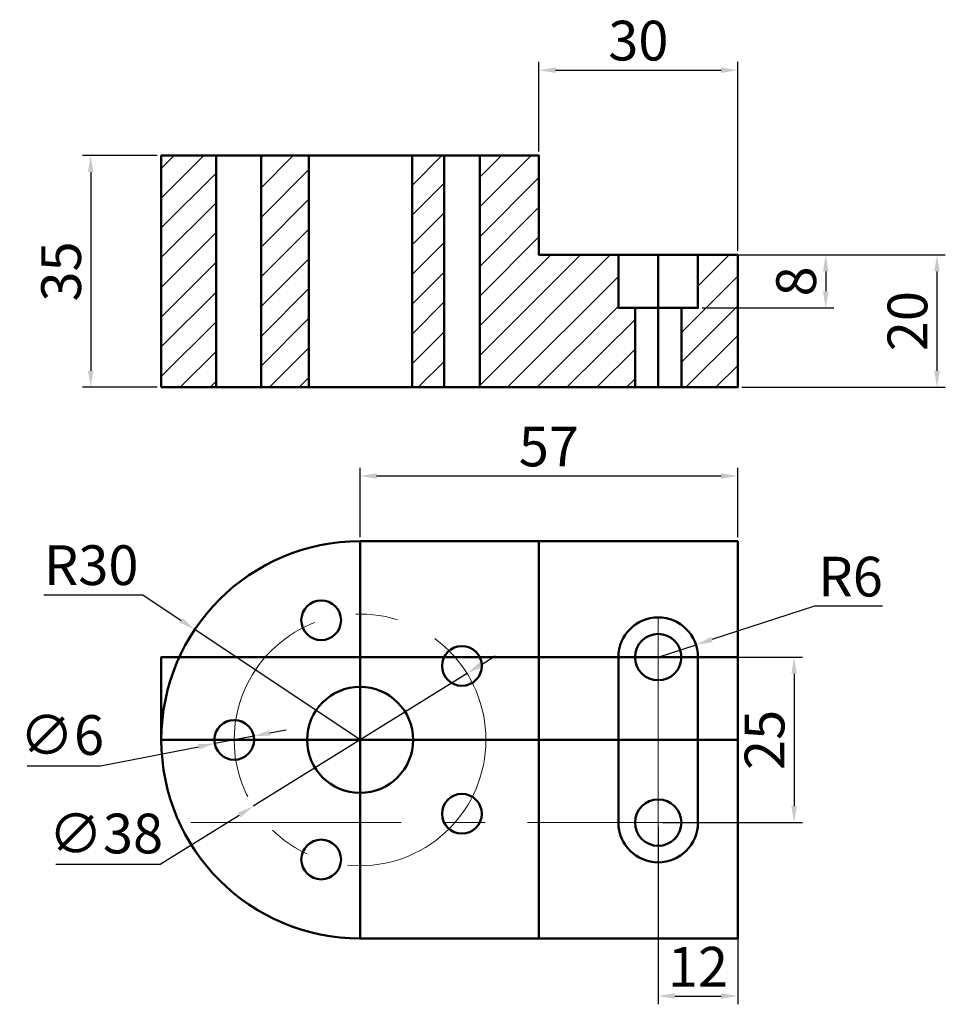
# Model space of a CAD drawing. Units: millimetres. Extents: x 3 to 142, y 5 to 154.
import ezdxf

# ---------------------------------------------------------------- set-up
doc = ezdxf.new("R2010")
doc.units = ezdxf.units.MM
doc.linetypes.add('CENTER', pattern=[50.8, 31.75, -6.35, 6.35, -6.35])
for name, color, linetype, lineweight in [('M-CNTR', 1, 'CENTER', 18), ('M-DIMS', 2, 'Continuous', 25), ('M-HATC', 8, 'Continuous', 18), ('M-OUTL', 7, 'Continuous', 50)]:
    doc.layers.add(name, color=color, linetype=linetype, lineweight=lineweight)
doc.styles.get("Standard").update_dxf_attribs({"font": 'arial.ttf'})
doc.dimstyles.new('ISO-25', dxfattribs={"dimtxt": 6, "dimasz": 2.5, "dimexe": 1.25, "dimexo": 0.625, "dimtad": 1, "dimtoh": 1, "dimdec": 0, "dimtxsty": 'Standard', "dimcen": 2.5, "dimadec": 0, "dimazin": 0, "dimtfac": 1, "dimtdec": 0, "dimtmove": 0, "dimatfit": 3, "dimfxl": 1, "dimarcsym": 0})

# ---------------------------------------------------------------- blocks, each defined once
blk = doc.blocks.new('*U1')
blk.add_circle((0, 0), 3)
blk = doc.blocks.new('*U2')
at = {"layer": 'M-OUTL', "color": 0, "linetype": 'ByBlock', "lineweight": -2, "transparency": 16777216}
for p, rotation in [((48.1, 63.49), 288), ((69.34, 56.59), 216), ((69.34, 34.26), 144), ((48.1, 27.35), 72.00000000000001)]:
    blk.add_blockref('*U1', p, dxfattribs=dict(at, rotation=rotation))
blk.add_blockref('*U1', (34.97, 45.42), dxfattribs=at)
blk = doc.blocks.new('*D3')
at = {"layer": 'Defpoints', "color": 0, "transparency": 16777216}
for p in [(23.97, 133.67), (13.31, 98.67), (23.97, 98.67)]:
    blk.add_point(p, dxfattribs=at)
at = {"layer": 'M-DIMS', "color": 0, "lineweight": -2, "transparency": 16777216}
for p, q in [((23.35, 133.67), (12.06, 133.67)), ((13.31, 131.17), (13.31, 101.17)), ((23.35, 98.67), (12.06, 98.67))]:
    blk.add_line(p, q, dxfattribs=at)
at = {"layer": 'M-DIMS', "color": 0, "transparency": 16777216}
for points in [[(12.89, 131.17), (13.72, 131.17), (13.31, 133.67)], [(12.89, 101.17), (13.72, 101.17), (13.31, 98.67)]]:
    blk.add_solid(points, dxfattribs=at)
at = {"layer": 'M-DIMS', "color": 0, "transparency": 16777216, "insert": (9.62, 116.17), "char_height": 6, "attachment_point": 5, "rotation": 90}
blk.add_mtext('35', dxfattribs=at)
blk = doc.blocks.new('*D4')
at = {"layer": 'Defpoints', "color": 0, "transparency": 16777216}
for p in [(110.97, 146.57), (80.97, 133.67), (110.97, 118.67)]:
    blk.add_point(p, dxfattribs=at)
at = {"layer": 'M-DIMS', "color": 0, "lineweight": -2, "transparency": 16777216}
for p, q in [((80.97, 134.29), (80.97, 147.82)), ((110.97, 119.29), (110.97, 147.82)), ((83.47, 146.57), (108.47, 146.57))]:
    blk.add_line(p, q, dxfattribs=at)
at = {"layer": 'M-DIMS', "color": 0, "transparency": 16777216}
for points in [[(83.47, 146.99), (83.47, 146.15), (80.97, 146.57)], [(108.47, 146.99), (108.47, 146.15), (110.97, 146.57)]]:
    blk.add_solid(points, dxfattribs=at)
at = {"layer": 'M-DIMS', "color": 0, "transparency": 16777216, "insert": (95.97, 150.26), "char_height": 6, "attachment_point": 5}
blk.add_mtext('30', dxfattribs=at)
blk = doc.blocks.new('*D5')
at = {"layer": 'Defpoints', "color": 0, "transparency": 16777216}
for p in [(104.97, 118.67), (104.97, 110.67), (124.25, 110.67)]:
    blk.add_point(p, dxfattribs=at)
at = {"layer": 'M-DIMS', "color": 0, "lineweight": -2, "transparency": 16777216}
for p, q in [((105.6, 118.67), (125.5, 118.67)), ((124.25, 116.17), (124.25, 113.17)), ((105.6, 110.67), (125.5, 110.67))]:
    blk.add_line(p, q, dxfattribs=at)
at = {"layer": 'M-DIMS', "color": 0, "transparency": 16777216}
for points in [[(123.84, 116.17), (124.67, 116.17), (124.25, 118.67)], [(123.84, 113.17), (124.67, 113.17), (124.25, 110.67)]]:
    blk.add_solid(points, dxfattribs=at)
at = {"layer": 'M-DIMS', "color": 0, "transparency": 16777216, "insert": (120.57, 114.67), "char_height": 6, "attachment_point": 5, "rotation": 90}
blk.add_mtext('8', dxfattribs=at)
blk = doc.blocks.new('*D6')
at = {"layer": 'Defpoints', "color": 0, "transparency": 16777216}
for p in [(110.97, 118.67), (110.97, 98.67), (141.05, 98.67)]:
    blk.add_point(p, dxfattribs=at)
at = {"layer": 'M-DIMS', "color": 0, "lineweight": -2, "transparency": 16777216}
for p, q in [((111.6, 118.67), (142.3, 118.67)), ((141.05, 116.17), (141.05, 101.17)), ((111.6, 98.67), (142.3, 98.67))]:
    blk.add_line(p, q, dxfattribs=at)
at = {"layer": 'M-DIMS', "color": 0, "transparency": 16777216}
for points in [[(140.64, 116.17), (141.47, 116.17), (141.05, 118.67)], [(140.64, 101.17), (141.47, 101.17), (141.05, 98.67)]]:
    blk.add_solid(points, dxfattribs=at)
at = {"layer": 'M-DIMS', "color": 0, "transparency": 16777216, "insert": (137.37, 108.67), "char_height": 6, "attachment_point": 5, "rotation": 90}
blk.add_mtext('20', dxfattribs=at)
blk = doc.blocks.new('*D7')
at = {"layer": 'Defpoints', "color": 0, "transparency": 16777216}
for p in [(104.68, 59.78), (98.97, 57.92)]:
    blk.add_point(p, dxfattribs=at)
at = {"layer": 'M-DIMS', "color": 0, "lineweight": -2, "transparency": 16777216}
for p, q in [((122.55, 65.61), (107.05, 60.56)), ((132.85, 65.61), (122.55, 65.61)), ((98.97, 57.92), (104.68, 59.78))]:
    blk.add_line(p, q, dxfattribs=at)
at = {"layer": 'M-DIMS', "color": 0, "transparency": 16777216}
blk.add_solid([(106.93, 60.96), (107.18, 60.16), (104.68, 59.78)], dxfattribs=at)
at = {"layer": 'M-DIMS', "color": 0, "transparency": 16777216, "insert": (128.01, 69.3), "char_height": 6, "attachment_point": 5}
blk.add_mtext('R6', dxfattribs=at)
blk = doc.blocks.new('*D8')
at = {"layer": 'Defpoints', "color": 0, "transparency": 16777216}
for p in [(98.97, 57.92), (98.97, 32.92), (119.48, 32.92)]:
    blk.add_point(p, dxfattribs=at)
at = {"layer": 'M-DIMS', "color": 0, "lineweight": -2, "transparency": 16777216}
for p, q in [((99.6, 57.92), (120.73, 57.92)), ((119.48, 55.42), (119.48, 35.42)), ((99.6, 32.92), (120.73, 32.92))]:
    blk.add_line(p, q, dxfattribs=at)
at = {"layer": 'M-DIMS', "color": 0, "transparency": 16777216}
for points in [[(119.07, 55.42), (119.9, 55.42), (119.48, 57.92)], [(119.07, 35.42), (119.9, 35.42), (119.48, 32.92)]]:
    blk.add_solid(points, dxfattribs=at)
at = {"layer": 'M-DIMS', "color": 0, "transparency": 16777216, "insert": (115.8, 45.42), "char_height": 6, "attachment_point": 5, "rotation": 90}
blk.add_mtext('25', dxfattribs=at)
blk = doc.blocks.new('*D9')
at = {"layer": 'Defpoints', "color": 0, "transparency": 16777216}
for p in [(98.97, 32.92), (110.97, 32.92), (110.97, 6.73)]:
    blk.add_point(p, dxfattribs=at)
at = {"layer": 'M-DIMS', "color": 0, "lineweight": -2, "transparency": 16777216}
for p, q in [((98.97, 32.3), (98.97, 5.48)), ((110.97, 32.3), (110.97, 5.48)), ((101.47, 6.73), (108.47, 6.73))]:
    blk.add_line(p, q, dxfattribs=at)
at = {"layer": 'M-DIMS', "color": 0, "transparency": 16777216}
for points in [[(101.47, 7.15), (101.47, 6.31), (98.97, 6.73)], [(108.47, 7.15), (108.47, 6.31), (110.97, 6.73)]]:
    blk.add_solid(points, dxfattribs=at)
at = {"layer": 'M-DIMS', "color": 0, "transparency": 16777216, "insert": (104.97, 10.37), "char_height": 6, "attachment_point": 5}
blk.add_mtext('12', dxfattribs=at)
blk = doc.blocks.new('*D10')
at = {"layer": 'Defpoints', "color": 0, "transparency": 16777216}
for p in [(110.97, 85.28), (53.97, 75.42), (110.97, 75.42)]:
    blk.add_point(p, dxfattribs=at)
at = {"layer": 'M-DIMS', "color": 0, "lineweight": -2, "transparency": 16777216}
for p, q in [((53.97, 76.05), (53.97, 86.53)), ((110.97, 76.05), (110.97, 86.53)), ((56.47, 85.28), (108.47, 85.28))]:
    blk.add_line(p, q, dxfattribs=at)
at = {"layer": 'M-DIMS', "color": 0, "transparency": 16777216}
for points in [[(56.47, 85.7), (56.47, 84.86), (53.97, 85.28)], [(108.47, 85.7), (108.47, 84.86), (110.97, 85.28)]]:
    blk.add_solid(points, dxfattribs=at)
at = {"layer": 'M-DIMS', "color": 0, "transparency": 16777216, "insert": (82.47, 88.96), "char_height": 6, "attachment_point": 5}
blk.add_mtext('57', dxfattribs=at)
blk = doc.blocks.new('*D11')
at = {"layer": 'Defpoints', "color": 0, "transparency": 16777216}
for p in [(29.03, 62.09), (53.97, 45.42)]:
    blk.add_point(p, dxfattribs=at)
at = {"layer": 'M-DIMS', "color": 0, "lineweight": -2, "transparency": 16777216}
for p, q in [((6.22, 67.34), (21.16, 67.34)), ((21.16, 67.34), (26.95, 63.47)), ((53.97, 45.42), (29.03, 62.09))]:
    blk.add_line(p, q, dxfattribs=at)
at = {"layer": 'M-DIMS', "color": 0, "transparency": 16777216}
blk.add_solid([(27.18, 63.82), (26.72, 63.13), (29.03, 62.09)], dxfattribs=at)
at = {"layer": 'M-DIMS', "color": 0, "transparency": 16777216, "insert": (13.38, 71.03), "char_height": 6, "attachment_point": 5}
blk.add_mtext('R30', dxfattribs=at)
blk = doc.blocks.new('*D12')
at = {"layer": 'Defpoints', "color": 0, "transparency": 16777216}
for p in [(32.03, 44.85), (37.92, 45.99)]:
    blk.add_point(p, dxfattribs=at)
at = {"layer": 'M-DIMS', "color": 0, "lineweight": -2, "transparency": 16777216}
for p, q in [((40.37, 46.47), (42.83, 46.95)), ((37.92, 45.99), (32.03, 44.85)), ((14.81, 41.52), (29.57, 44.38)), ((3.73, 41.52), (14.81, 41.52))]:
    blk.add_line(p, q, dxfattribs=at)
at = {"layer": 'M-DIMS', "color": 0, "transparency": 16777216}
for points in [[(40.29, 46.88), (40.45, 46.06), (37.92, 45.99)], [(29.49, 44.79), (29.65, 43.97), (32.03, 44.85)]]:
    blk.add_solid(points, dxfattribs=at)
at = {"layer": 'M-DIMS', "color": 0, "transparency": 16777216, "insert": (8.96, 45.38), "char_height": 6, "attachment_point": 5}
blk.add_mtext('∅6', dxfattribs=at)
blk = doc.blocks.new('*D13')
at = {"layer": 'Defpoints', "color": 0, "transparency": 16777216}
for p in [(70.11, 55.46), (37.84, 35.39)]:
    blk.add_point(p, dxfattribs=at)
at = {"layer": 'M-DIMS', "color": 0, "lineweight": -2, "transparency": 16777216}
for p, q in [((72.23, 56.78), (74.35, 58.1)), ((70.11, 55.46), (37.84, 35.39)), ((23.79, 26.64), (35.72, 34.07)), ((8.03, 26.64), (23.79, 26.64))]:
    blk.add_line(p, q, dxfattribs=at)
at = {"layer": 'M-DIMS', "color": 0, "transparency": 16777216}
for points in [[(72.01, 57.14), (72.45, 56.43), (70.11, 55.46)], [(35.5, 34.42), (35.94, 33.71), (37.84, 35.39)]]:
    blk.add_solid(points, dxfattribs=at)
at = {"layer": 'M-DIMS', "color": 0, "transparency": 16777216, "insert": (15.6, 30.5), "char_height": 6, "attachment_point": 5}
blk.add_mtext('∅38', dxfattribs=at)

msp = doc.modelspace()

# ---------------------------------------------------------------- hatches: boundary and pattern name
at = {"layer": 'M-HATC'}
h = msp.add_hatch(dxfattribs=at)
h.set_pattern_fill('ANSI31', color=256)
h.paths.add_polyline_path([(32.24, 133.67), (23.97, 133.67), (23.97, 98.67), (32.24, 98.67)])
h.paths.add_polyline_path([(46.25, 133.67), (39.02, 133.67), (39.02, 98.67), (46.25, 98.67)])
h.paths.add_polyline_path([(66.66, 133.67), (61.82, 133.67), (61.82, 98.67), (66.66, 98.67)])
h.paths.add_polyline_path([(80.97, 133.67), (72.03, 133.67), (72.03, 98.67), (95.47, 98.67), (95.47, 110.67), (92.97, 110.67), (92.97, 118.67), (80.97, 118.67)])
h.paths.add_polyline_path([(110.97, 118.67), (104.97, 118.67), (104.97, 110.67), (102.47, 110.67), (102.47, 98.67), (110.97, 98.67)])

# ---------------------------------------------------------------- linework, layer by layer
at = {"layer": 'M-CNTR'}
for p, q in [((98.97, 63.92), (98.97, 15.42)), ((110.97, 32.92), (23.97, 32.92))]:
    msp.add_line(p, q, dxfattribs=at)
msp.add_circle((53.97, 45.42), 19, dxfattribs=at)
at = {"layer": 'M-OUTL'}
for p, q in [((32.24, 98.67), (32.24, 133.67)), ((39.02, 98.67), (39.02, 133.67)), ((46.25, 98.67), (46.25, 133.67)), ((61.82, 98.67), (61.82, 133.67)), ((66.66, 98.67), (66.66, 133.67)), ((72.03, 98.67), (72.03, 133.67)), ((98.97, 118.67), (98.97, 98.67)), ((95.47, 98.67), (95.47, 110.67)), ((102.47, 98.67), (102.47, 110.67)), ((80.97, 75.42), (80.97, 15.42))]:
    msp.add_line(p, q, dxfattribs=at)
for points in [[(23.97, 98.67), (23.97, 133.67), (80.97, 133.67), (80.97, 118.67), (110.97, 118.67), (110.97, 98.67)], [(110.97, 75.42), (110.97, 15.42), (53.97, 15.42), (53.97, 75.42)]]:
    msp.add_lwpolyline(points, close=True, dxfattribs=at)
for points in [[(92.97, 118.67), (92.97, 110.67), (104.97, 110.67), (104.97, 118.67)], [(110.97, 45.42), (23.97, 45.42), (23.97, 57.92), (110.97, 57.92)]]:
    msp.add_lwpolyline(points, dxfattribs=at)
msp.add_lwpolyline([(104.97, 57.92), (104.97, 32.92, -1), (92.97, 32.92), (92.97, 57.92, -1)], format="xyb", close=True, dxfattribs=at)
for centre, radius in [((98.97, 57.92), 3.5), ((53.97, 45.42), 8), ((98.97, 32.92), 3.5)]:
    msp.add_circle(centre, radius, dxfattribs=at)
msp.add_arc((53.97, 45.42), 30, 90, 270, dxfattribs=at)

# ---------------------------------------------------------------- block references
msp.add_blockref('*U2', (0, 0), dxfattribs=at)

# ---------------------------------------------------------------- dimensions: what is measured, and where the dimension line sits
at = {"layer": 'M-DIMS'}
for base, p1, p2, picture, middle in [((110.97, 146.57), (80.97, 133.67), (110.97, 118.67), '*D4', (95.97, 150.26)), ((110.97, 85.28), (53.97, 75.42), (110.97, 75.42), '*D10', (82.47, 88.96)), ((110.97, 6.73), (98.97, 32.92), (110.97, 32.92), '*D9', (104.97, 10.37))]:
    dim = msp.add_linear_dim(base=base, p1=p1, p2=p2, dimstyle='ISO-25', override={"dimclrd": 0, "dimclre": 0, "dimclrt": 0}, dxfattribs=at)
    dim.commit()
    dim.dimension.update_dxf_attribs({"geometry": picture, "text_midpoint": middle})
for base, p1, p2, picture, middle in [((13.31, 98.67), (23.97, 133.67), (23.97, 98.67), '*D3', (9.62, 116.17)), ((124.25, 110.67), (104.97, 118.67), (104.97, 110.67), '*D5', (120.57, 114.67)), ((141.05, 98.67), (110.97, 118.67), (110.97, 98.67), '*D6', (137.37, 108.67)), ((119.48, 32.92), (98.97, 57.92), (98.97, 32.92), '*D8', (115.8, 45.42))]:
    dim = msp.add_linear_dim(base=base, p1=p1, p2=p2, angle=90, dimstyle='ISO-25', override={"dimclrd": 0, "dimclre": 0, "dimclrt": 0}, dxfattribs=at)
    dim.commit()
    dim.dimension.update_dxf_attribs({"geometry": picture, "text_midpoint": middle})
for center, mpoint, picture, middle in [((53.97, 45.42), (29.03, 62.09), '*D11', (13.38, 67.34)), ((98.97, 57.92), (104.68, 59.78), '*D7', (128.01, 65.61))]:
    dim = msp.add_radius_dim(center=center, mpoint=mpoint, dimstyle='ISO-25', override={"dimclrd": 0, "dimclre": 0, "dimclrt": 0}, dxfattribs=at)
    dim.commit()
    dim.dimension.update_dxf_attribs({"geometry": picture, "text_midpoint": middle, "dimtype": 164})
for p1, p2, picture, middle in [((70.11, 55.46), (37.84, 35.39), '*D13', (15.6, 26.64)), ((37.92, 45.99), (32.03, 44.85), '*D12', (14.81, 41.52))]:
    dim = msp.add_diameter_dim_2p(p1=p1, p2=p2, dimstyle='ISO-25', override={"dimclrd": 0, "dimclre": 0, "dimclrt": 0}, dxfattribs=at)
    dim.commit()
    dim.dimension.update_dxf_attribs({"geometry": picture, "text_midpoint": middle, "dimtype": 163})

doc.saveas('drawing.dxf')
